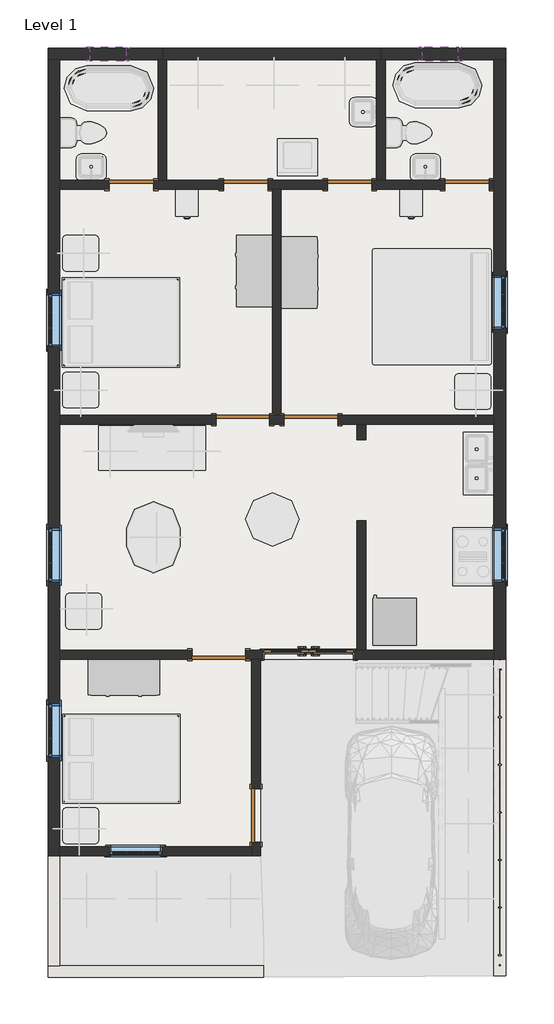
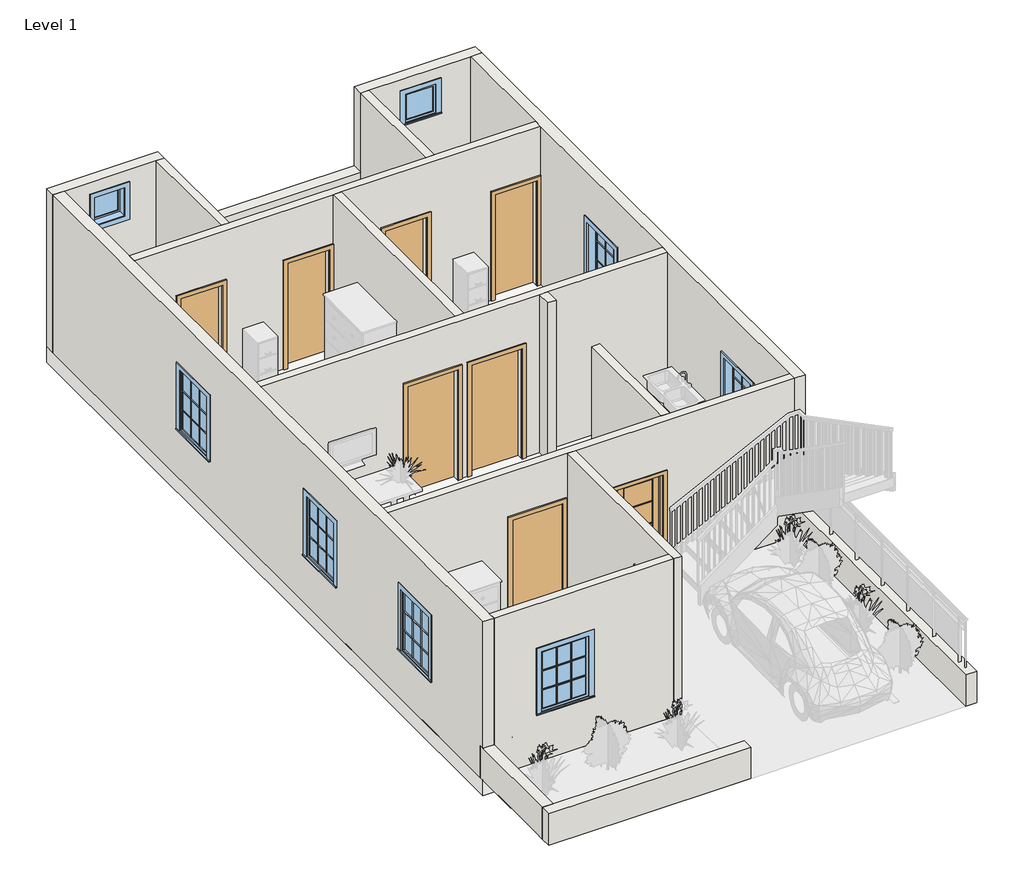
# One storey, part 1 of 3: 18 walls, 9 doors, 8 windows, 1 slab.
"""IFC4 building model written with IfcOpenShell, lengths in millimetres."""

from ifc_helpers import new_model, si_unit, frame, origin, origin_with_axes, place, context, project, spatial, polyline, outline, extrude, faceted_brep, transform, mapped, element, save
from components import door_94998e6c, door_059fdd7e, door_16372e1c, door_686f89d2, window_29c06734, window_5c190c7e, window_e41d21a6

model = new_model("IFC4")

# Units and contexts
model_context = context("Model", 3, world=origin())
ifc_project = project(units=[si_unit("LENGTHUNIT", "METRE", prefix="MILLI")], contexts=[model_context])

# Site, building, storey
site = spatial("IfcSite", under=ifc_project)
building = spatial("IfcBuilding", under=site)
storey = spatial("IfcBuildingStorey", under=building, Name="Level 1", Elevation=0.0)

# Doors
placement = place(None, origin())
door_shape = door_94998e6c(model_context)
element("IfcDoor", 1, ObjectType="Door-Exterior-Double-Full Glass-Wood_Clad : 60\" x 80\"", at=placement, inside=storey, context=model_context, shape_type="MappedRepresentation", body=[
    mapped(door_shape, transform((1366.1339716, 319.025395, 0.0), x_axis=(1.0, 0.0, 0.0), y_axis=(0.0, 1.0, 0.0), z_axis=(0.0, 0.0, 1.0))),
])
door_2_shape = door_059fdd7e(model_context)
element("IfcDoor", 2, ObjectType="Single-Flush : 30\" x 80\"", at=placement, inside=storey, context=model_context, shape_type="MappedRepresentation", body=[
    mapped(door_2_shape, transform((-1669.1660284, 8342.250395, 0.0), x_axis=(1.0, 0.0, 0.0), y_axis=(0.0, 1.0, 0.0), z_axis=(0.0, 0.0, 1.0))),
])
element("IfcDoor", 3, ObjectType="Single-Flush : 30\" x 80\"", at=placement, inside=storey, context=model_context, shape_type="MappedRepresentation", body=[
    mapped(door_2_shape, transform((286.6339716, 8342.250395, 0.0), x_axis=(1.0, 0.0, 0.0), y_axis=(0.0, 1.0, 0.0), z_axis=(0.0, 0.0, 1.0))),
])
element("IfcDoor", 4, ObjectType="Single-Flush : 30\" x 80\"", at=placement, inside=storey, context=model_context, shape_type="MappedRepresentation", body=[
    mapped(door_2_shape, transform((2064.6339716, 8342.250395, 0.0), x_axis=(1.0, 0.0, 0.0), y_axis=(0.0, 1.0, 0.0), z_axis=(0.0, 0.0, 1.0))),
])
element("IfcDoor", 5, ObjectType="Single-Flush : 30\" x 80\"", at=placement, inside=storey, context=model_context, shape_type="MappedRepresentation", body=[
    mapped(door_2_shape, transform((4071.2339716, 8342.250395, 0.0), x_axis=(1.0, 0.0, 0.0), y_axis=(0.0, 1.0, 0.0), z_axis=(0.0, 0.0, 1.0))),
])
door_3_shape = door_16372e1c(model_context)
element("IfcDoor", 6, ObjectType="Single-Flush : 36\" x 84\"", at=placement, inside=storey, context=model_context, shape_type="MappedRepresentation", body=[
    mapped(door_3_shape, transform((235.8339716, 4329.050395, 0.0), x_axis=(1.0, 0.0, 0.0), y_axis=(0.0, 1.0, 0.0), z_axis=(0.0, 0.0, 1.0))),
])
door_4_shape = door_686f89d2(model_context)
element("IfcDoor", 7, ObjectType="Single-Flush : 36\" x 84\"", at=placement, inside=storey, context=model_context, shape_type="MappedRepresentation", body=[
    mapped(door_4_shape, transform((1404.2339716, 4329.050395, 0.0), x_axis=(-1.0, 0.0, 0.0), y_axis=(0.0, -1.0, 0.0), z_axis=(0.0, 0.0, 1.0))),
])
element("IfcDoor", 8, ObjectType="Single-Flush : 36\" x 84\"", at=placement, inside=storey, context=model_context, shape_type="MappedRepresentation", body=[
    mapped(door_4_shape, transform((-170.5660284, 315.850395, 0.0), x_axis=(1.0, 0.0, 0.0), y_axis=(0.0, 1.0, 0.0), z_axis=(0.0, 0.0, 1.0))),
])
element("IfcDoor", 9, ObjectType="Single-Flush : 36\" x 84\"", at=placement, inside=storey, context=model_context, shape_type="MappedRepresentation", body=[
    mapped(door_4_shape, transform((464.4339716, -2427.349605, 0.0), x_axis=(0.0, -1.0, 0.0), y_axis=(1.0, 0.0, 0.0), z_axis=(0.0, 0.0, 1.0))),
])

# Slab
element("IfcSlab", 10, ObjectType="Generic - 12\"", at=placement, inside=storey, context=model_context, shape_type="SweptSolid", body=[
    extrude(outline(polyline([(4731.6339716, 10679.050395), (4731.6339716, 239.650395), (540.6339716, 239.650395), (540.6339716, -3113.149605), (-3091.5660284, -3113.149605), (-3091.5660284, 10679.050395), (4731.6339716, 10679.050395)])), frame((0.0, 0.0, -304.8), z_axis=(0.0, 0.0, 1.0), x_axis=(1.0, 0.0, 0.0)), (0.0, 0.0, 1.0), 304.8),
])

# Walls
element("IfcWall", 11, ObjectType="Generic - 2'", at=placement, inside=storey, context=model_context, shape_type="Brep", body=[
    faceted_brep([(4528.4339716, 315.850395, 0.0), (4528.4339716, 239.650395, 0.0), (4528.4339716, -5170.549605, 0.0), (4528.4339716, -5170.549605, 609.6), (4528.4339716, 315.850395, 609.6), (4731.6339716, 315.850395, 0.0), (4731.6339716, 315.850395, 609.6), (4731.6339716, -5170.549605, 609.6), (4731.6339716, -5170.549605, 0.0)], [[[0, 1, 2, 3, 4]], [[5, 6, 7, 8]], [[2, 1, 0, 5, 8]], [[3, 2, 8, 7]], [[4, 3, 7, 6]], [[0, 4, 6, 5]]]),
])
element("IfcWall", 12, ObjectType="Generic - 2'", at=placement, inside=storey, context=model_context, shape_type="Brep", body=[
    faceted_brep([(591.4339716, -4992.749605, 0.0), (-2888.3660284, -4992.749605, 0.0), (-3091.5660284, -4992.749605, 0.0), (-3091.5660284, -4992.749605, 609.6), (-2888.3660284, -4992.749605, 609.6), (591.4339716, -4992.749605, 609.6), (591.4339716, -5195.949605, 0.0), (591.4339716, -5195.949605, 609.6), (-3091.5660284, -5195.949605, 609.6), (-3091.5660284, -5195.949605, 0.0)], [[[0, 1, 2, 3, 4, 5]], [[6, 7, 8, 9]], [[2, 1, 0, 6, 9]], [[5, 4, 3, 8, 7]], [[0, 5, 7, 6]], [[3, 2, 9, 8]]]),
])
element("IfcWall", 13, ObjectType="Generic - 8\"", at=placement, inside=storey, context=model_context, shape_type="Brep", body=[
    faceted_brep([(-3091.5660284, 10475.850395, 0.0), (-2888.3660284, 10475.850395, 0.0), (-1211.9660284, 10475.850395, 0.0), (-1135.7660284, 10475.850395, 0.0), (-1135.7660284, 10475.850395, 1524.0), (-1059.5660284, 10475.850395, 1524.0), (-1059.5660284, 10475.850395, 3048.0), (-1211.9660284, 10475.850395, 3048.0), (-2888.3660284, 10475.850395, 3048.0), (-3091.5660284, 10475.850395, 3048.0), (-1758.0660284, 10475.850395, 2768.6), (-1758.0660284, 10475.850395, 2159.0), (-2367.6660284, 10475.850395, 2159.0), (-2367.6660284, 10475.850395, 2768.6), (-3091.5660284, 10679.050395, 0.0), (-3091.5660284, 10679.050395, 3048.0), (-1059.5660284, 10679.050395, 3048.0), (-1059.5660284, 10679.050395, 1524.0), (-1135.7660284, 10679.050395, 1524.0), (-1135.7660284, 10679.050395, 0.0), (-1758.0660284, 10679.050395, 2768.6), (-2367.6660284, 10679.050395, 2768.6), (-2367.6660284, 10679.050395, 2159.0), (-1758.0660284, 10679.050395, 2159.0)], [[[0, 1, 2, 3, 4, 5, 6, 7, 8, 9], [10, 11, 12, 13]], [[14, 15, 16, 17, 18, 19], [20, 21, 22, 23]], [[3, 2, 1, 0, 14, 19]], [[0, 9, 15, 14]], [[11, 10, 20, 23]], [[12, 11, 23, 22]], [[13, 12, 22, 21]], [[10, 13, 21, 20]], [[4, 3, 19, 18]], [[17, 5, 4, 18]], [[6, 5, 17, 16]], [[9, 8, 7, 6, 16, 15]]]),
])
element("IfcWall", 14, ObjectType="Generic - 8\"", at=placement, inside=storey, context=model_context, shape_type="Brep", body=[
    faceted_brep([(4528.4339716, 10475.850395, 0.0), (4528.4339716, 8418.450395, 0.0), (4528.4339716, 8266.050395, 0.0), (4528.4339716, 4405.250395, 0.0), (4528.4339716, 4252.850395, 0.0), (4528.4339716, 392.050395, 0.0), (4528.4339716, 315.850395, 0.0), (4528.4339716, 315.850395, 609.6), (4528.4339716, 239.650395, 609.6), (4528.4339716, 239.650395, 3048.0), (4528.4339716, 392.050395, 3048.0), (4528.4339716, 4252.850395, 3048.0), (4528.4339716, 4405.250395, 3048.0), (4528.4339716, 8266.050395, 3048.0), (4528.4339716, 8418.450395, 3048.0), (4528.4339716, 10475.850395, 3048.0), (4528.4339716, 5878.450395, 2133.6), (4528.4339716, 5878.450395, 914.4), (4528.4339716, 6792.850395, 914.4), (4528.4339716, 6792.850395, 2133.6), (4528.4339716, 1560.450395, 2133.6), (4528.4339716, 1560.450395, 914.4), (4528.4339716, 2474.850395, 914.4), (4528.4339716, 2474.850395, 2133.6), (4731.6339716, 10475.850395, 0.0), (4731.6339716, 10475.850395, 3048.0), (4731.6339716, 239.650395, 3048.0), (4731.6339716, 239.650395, 609.6), (4731.6339716, 315.850395, 609.6), (4731.6339716, 315.850395, 0.0), (4731.6339716, 5878.450395, 2133.6), (4731.6339716, 6792.850395, 2133.6), (4731.6339716, 6792.850395, 914.4), (4731.6339716, 5878.450395, 914.4), (4731.6339716, 1560.450395, 2133.6), (4731.6339716, 2474.850395, 2133.6), (4731.6339716, 2474.850395, 914.4), (4731.6339716, 1560.450395, 914.4)], [[[0, 1, 2, 3, 4, 5, 6, 7, 8, 9, 10, 11, 12, 13, 14, 15], [16, 17, 18, 19], [20, 21, 22, 23]], [[24, 25, 26, 27, 28, 29], [30, 31, 32, 33], [34, 35, 36, 37]], [[6, 5, 4, 3, 2, 1, 0, 24, 29]], [[0, 15, 25, 24]], [[7, 6, 29, 28]], [[27, 8, 7, 28]], [[9, 8, 27, 26]], [[17, 16, 30, 33]], [[18, 17, 33, 32]], [[19, 18, 32, 31]], [[16, 19, 31, 30]], [[21, 20, 34, 37]], [[22, 21, 37, 36]], [[23, 22, 36, 35]], [[20, 23, 35, 34]], [[15, 14, 13, 12, 11, 10, 9, 26, 25]]]),
])
element("IfcWall", 15, ObjectType="Generic - 8\"", at=placement, inside=storey, context=model_context, shape_type="Brep", body=[
    faceted_brep([(-2888.3660284, -4992.749605, 0.0), (-2888.3660284, -3113.149605, 0.0), (-2888.3660284, -3036.949605, 0.0), (-2888.3660284, -3036.949605, 609.6), (-2888.3660284, -3113.149605, 609.6), (-2888.3660284, -4992.749605, 609.6), (-3091.5660284, -4992.749605, 0.0), (-3091.5660284, -4992.749605, 609.6), (-3091.5660284, -3113.149605, 609.6), (-3091.5660284, -3036.949605, 609.6), (-3091.5660284, -3036.949605, 0.0)], [[[0, 1, 2, 3, 4, 5]], [[6, 7, 8, 9, 10]], [[2, 1, 0, 6, 10]], [[3, 2, 10, 9]], [[5, 4, 3, 9, 8, 7]], [[0, 5, 7, 6]]]),
])
element("IfcWall", 16, ObjectType="Generic - 8\"", at=placement, inside=storey, context=model_context, shape_type="Brep", body=[
    faceted_brep([(-2888.3660284, -3036.949605, 0.0), (-2888.3660284, -2960.749605, 0.0), (-2888.3660284, 239.650395, 0.0), (-2888.3660284, 392.050395, 0.0), (-2888.3660284, 4252.850395, 0.0), (-2888.3660284, 4405.250395, 0.0), (-2888.3660284, 8266.050395, 0.0), (-2888.3660284, 8418.450395, 0.0), (-2888.3660284, 10475.850395, 0.0), (-2888.3660284, 10475.850395, 3048.0), (-2888.3660284, 8418.450395, 3048.0), (-2888.3660284, 8266.050395, 3048.0), (-2888.3660284, 4405.250395, 3048.0), (-2888.3660284, 4252.850395, 3048.0), (-2888.3660284, 392.050395, 3048.0), (-2888.3660284, 239.650395, 3048.0), (-2888.3660284, -2960.749605, 3048.0), (-2888.3660284, -3113.149605, 3048.0), (-2888.3660284, -3113.149605, 609.6), (-2888.3660284, -3036.949605, 609.6), (-2888.3660284, 6488.050395, 2133.6), (-2888.3660284, 6488.050395, 914.4), (-2888.3660284, 5573.650395, 914.4), (-2888.3660284, 5573.650395, 2133.6), (-2888.3660284, 2474.850395, 2133.6), (-2888.3660284, 2474.850395, 914.4), (-2888.3660284, 1560.450395, 914.4), (-2888.3660284, 1560.450395, 2133.6), (-2888.3660284, -522.349605, 2133.6), (-2888.3660284, -522.349605, 914.4), (-2888.3660284, -1436.749605, 914.4), (-2888.3660284, -1436.749605, 2133.6), (-3091.5660284, -3036.949605, 0.0), (-3091.5660284, -3036.949605, 609.6), (-3091.5660284, -3113.149605, 609.6), (-3091.5660284, -3113.149605, 3048.0), (-3091.5660284, 10475.850395, 3048.0), (-3091.5660284, 10475.850395, 0.0), (-3091.5660284, 6488.050395, 2133.6), (-3091.5660284, 5573.650395, 2133.6), (-3091.5660284, 5573.650395, 914.4), (-3091.5660284, 6488.050395, 914.4), (-3091.5660284, 2474.850395, 2133.6), (-3091.5660284, 1560.450395, 2133.6), (-3091.5660284, 1560.450395, 914.4), (-3091.5660284, 2474.850395, 914.4), (-3091.5660284, -522.349605, 2133.6), (-3091.5660284, -1436.749605, 2133.6), (-3091.5660284, -1436.749605, 914.4), (-3091.5660284, -522.349605, 914.4)], [[[0, 1, 2, 3, 4, 5, 6, 7, 8, 9, 10, 11, 12, 13, 14, 15, 16, 17, 18, 19], [20, 21, 22, 23], [24, 25, 26, 27], [28, 29, 30, 31]], [[32, 33, 34, 35, 36, 37], [38, 39, 40, 41], [42, 43, 44, 45], [46, 47, 48, 49]], [[8, 7, 6, 5, 4, 3, 2, 1, 0, 32, 37]], [[9, 8, 37, 36]], [[0, 19, 33, 32]], [[18, 34, 33, 19]], [[18, 17, 35, 34]], [[21, 20, 38, 41]], [[22, 21, 41, 40]], [[23, 22, 40, 39]], [[20, 23, 39, 38]], [[25, 24, 42, 45]], [[26, 25, 45, 44]], [[27, 26, 44, 43]], [[24, 27, 43, 42]], [[29, 28, 46, 49]], [[30, 29, 49, 48]], [[31, 30, 48, 47]], [[28, 31, 47, 46]], [[17, 16, 15, 14, 13, 12, 11, 10, 9, 36, 35]]]),
])
element("IfcWall", 17, ObjectType="Generic - 8\"", at=placement, inside=storey, context=model_context, shape_type="Brep", body=[
    faceted_brep([(2598.0339716, 10475.850395, 0.0), (2674.2339716, 10475.850395, 0.0), (4528.4339716, 10475.850395, 0.0), (4731.6339716, 10475.850395, 0.0), (4731.6339716, 10475.850395, 3048.0), (4528.4339716, 10475.850395, 3048.0), (2674.2339716, 10475.850395, 3048.0), (2521.8339716, 10475.850395, 3048.0), (2521.8339716, 10475.850395, 1524.0), (2598.0339716, 10475.850395, 1524.0), (3309.2339716, 10475.850395, 2768.6), (3918.8339716, 10475.850395, 2768.6), (3918.8339716, 10475.850395, 2159.0), (3309.2339716, 10475.850395, 2159.0), (2598.0339716, 10679.050395, 0.0), (2598.0339716, 10679.050395, 1524.0), (2521.8339716, 10679.050395, 1524.0), (2521.8339716, 10679.050395, 3048.0), (4731.6339716, 10679.050395, 3048.0), (4731.6339716, 10679.050395, 0.0), (3309.2339716, 10679.050395, 2768.6), (3309.2339716, 10679.050395, 2159.0), (3918.8339716, 10679.050395, 2159.0), (3918.8339716, 10679.050395, 2768.6)], [[[0, 1, 2, 3, 4, 5, 6, 7, 8, 9], [10, 11, 12, 13]], [[14, 15, 16, 17, 18, 19], [20, 21, 22, 23]], [[3, 2, 1, 0, 14, 19]], [[4, 3, 19, 18]], [[20, 23, 11, 10]], [[23, 22, 12, 11]], [[22, 21, 13, 12]], [[21, 20, 10, 13]], [[0, 9, 15, 14]], [[8, 16, 15, 9]], [[8, 7, 17, 16]], [[7, 6, 5, 4, 18, 17]]]),
])
element("IfcWall", 18, ObjectType="Generic - 8\"", at=placement, inside=storey, context=model_context, shape_type="Brep", body=[
    faceted_brep([(-1135.7660284, 10475.850395, 0.0), (-1059.5660284, 10475.850395, 0.0), (2521.8339716, 10475.850395, 0.0), (2598.0339716, 10475.850395, 0.0), (2598.0339716, 10475.850395, 1524.0), (2521.8339716, 10475.850395, 1524.0), (-1059.5660284, 10475.850395, 1524.0), (-1135.7660284, 10475.850395, 1524.0), (-1135.7660284, 10679.050395, 0.0), (-1135.7660284, 10679.050395, 1524.0), (-1059.5660284, 10679.050395, 1524.0), (2521.8339716, 10679.050395, 1524.0), (2598.0339716, 10679.050395, 1524.0), (2598.0339716, 10679.050395, 0.0)], [[[0, 1, 2, 3, 4, 5, 6, 7]], [[8, 9, 10, 11, 12, 13]], [[3, 2, 1, 0, 8, 13]], [[4, 3, 13, 12]], [[7, 6, 5, 4, 12, 11, 10, 9]], [[0, 7, 9, 8]]]),
])
element("IfcWall", 19, ObjectType="INNER 6\"", at=placement, inside=storey, context=model_context, shape_type="Brep", body=[
    faceted_brep([(4452.2339716, 8266.050395, 2032.0), (4452.2339716, 8266.050395, 0.0), (4528.4339716, 8266.050395, 0.0), (4528.4339716, 8266.050395, 3048.0), (896.2339716, 8266.050395, 3048.0), (743.8339716, 8266.050395, 3048.0), (-2888.3660284, 8266.050395, 3048.0), (-2888.3660284, 8266.050395, 0.0), (-2050.1660284, 8266.050395, 0.0), (-2050.1660284, 8266.050395, 2032.0), (-1288.1660284, 8266.050395, 2032.0), (-1288.1660284, 8266.050395, 0.0), (-94.3660284, 8266.050395, 0.0), (-94.3660284, 8266.050395, 2032.0), (667.6339716, 8266.050395, 2032.0), (667.6339716, 8266.050395, 0.0), (743.8339716, 8266.050395, 0.0), (896.2339716, 8266.050395, 0.0), (1683.6339716, 8266.050395, 0.0), (1683.6339716, 8266.050395, 2032.0), (2445.6339716, 8266.050395, 2032.0), (2445.6339716, 8266.050395, 0.0), (3690.2339716, 8266.050395, 0.0), (3690.2339716, 8266.050395, 2032.0), (4528.4339716, 8418.450395, 0.0), (4452.2339716, 8418.450395, 0.0), (4452.2339716, 8418.450395, 2032.0), (3690.2339716, 8418.450395, 2032.0), (3690.2339716, 8418.450395, 0.0), (2674.2339716, 8418.450395, 0.0), (2521.8339716, 8418.450395, 0.0), (2445.6339716, 8418.450395, 0.0), (2445.6339716, 8418.450395, 2032.0), (1683.6339716, 8418.450395, 2032.0), (1683.6339716, 8418.450395, 0.0), (667.6339716, 8418.450395, 0.0), (667.6339716, 8418.450395, 2032.0), (-94.3660284, 8418.450395, 2032.0), (-94.3660284, 8418.450395, 0.0), (-1059.5660284, 8418.450395, 0.0), (-1211.9660284, 8418.450395, 0.0), (-1288.1660284, 8418.450395, 0.0), (-1288.1660284, 8418.450395, 2032.0), (-2050.1660284, 8418.450395, 2032.0), (-2050.1660284, 8418.450395, 0.0), (-2888.3660284, 8418.450395, 0.0), (-2888.3660284, 8418.450395, 3048.0), (-1211.9660284, 8418.450395, 3048.0), (-1059.5660284, 8418.450395, 3048.0), (2521.8339716, 8418.450395, 3048.0), (2674.2339716, 8418.450395, 3048.0), (4528.4339716, 8418.450395, 3048.0)], [[[0, 1, 2, 3, 4, 5, 6, 7, 8, 9, 10, 11, 12, 13, 14, 15, 16, 17, 18, 19, 20, 21, 22, 23]], [[24, 25, 26, 27, 28, 29, 30, 31, 32, 33, 34, 35, 36, 37, 38, 39, 40, 41, 42, 43, 44, 45, 46, 47, 48, 49, 50, 51]], [[8, 7, 45, 44]], [[12, 11, 41, 40, 39, 38]], [[18, 17, 16, 15, 35, 34]], [[22, 21, 31, 30, 29, 28]], [[2, 1, 25, 24]], [[3, 2, 24, 51]], [[7, 6, 46, 45]], [[42, 41, 11, 10]], [[43, 42, 10, 9]], [[44, 43, 9, 8]], [[36, 35, 15, 14]], [[37, 36, 14, 13]], [[38, 37, 13, 12]], [[32, 31, 21, 20]], [[33, 32, 20, 19]], [[34, 33, 19, 18]], [[26, 25, 1, 0]], [[27, 26, 0, 23]], [[28, 27, 23, 22]], [[6, 5, 4, 3, 51, 50, 49, 48, 47, 46]]]),
])
element("IfcWall", 20, ObjectType="INNER 6\"", at=placement, inside=storey, context=model_context, shape_type="Brep", body=[
    faceted_brep([(693.0339716, 4252.850395, 0.0), (947.0339716, 4252.850395, 0.0), (947.0339716, 4252.850395, 2133.6), (1861.4339716, 4252.850395, 2133.6), (1861.4339716, 4252.850395, 0.0), (2191.6339716, 4252.850395, 0.0), (2344.0339716, 4252.850395, 0.0), (4528.4339716, 4252.850395, 0.0), (4528.4339716, 4252.850395, 3048.0), (2344.0339716, 4252.850395, 3048.0), (2191.6339716, 4252.850395, 3048.0), (-2888.3660284, 4252.850395, 3048.0), (-2888.3660284, 4252.850395, 0.0), (-221.3660284, 4252.850395, 0.0), (-221.3660284, 4252.850395, 2133.6), (693.0339716, 4252.850395, 2133.6), (947.0339716, 4405.250395, 2133.6), (947.0339716, 4405.250395, 0.0), (896.2339716, 4405.250395, 0.0), (743.8339716, 4405.250395, 0.0), (693.0339716, 4405.250395, 0.0), (693.0339716, 4405.250395, 2133.6), (-221.3660284, 4405.250395, 2133.6), (-221.3660284, 4405.250395, 0.0), (-2888.3660284, 4405.250395, 0.0), (-2888.3660284, 4405.250395, 3048.0), (743.8339716, 4405.250395, 3048.0), (896.2339716, 4405.250395, 3048.0), (4528.4339716, 4405.250395, 3048.0), (4528.4339716, 4405.250395, 0.0), (1861.4339716, 4405.250395, 0.0), (1861.4339716, 4405.250395, 2133.6)], [[[0, 1, 2, 3, 4, 5, 6, 7, 8, 9, 10, 11, 12, 13, 14, 15]], [[16, 17, 18, 19, 20, 21, 22, 23, 24, 25, 26, 27, 28, 29, 30, 31]], [[13, 12, 24, 23]], [[30, 29, 7, 6, 5, 4]], [[20, 19, 18, 17, 1, 0]], [[8, 7, 29, 28]], [[12, 11, 25, 24]], [[21, 20, 0, 15]], [[22, 21, 15, 14]], [[23, 22, 14, 13]], [[2, 1, 17, 16]], [[3, 2, 16, 31]], [[4, 3, 31, 30]], [[11, 10, 9, 8, 28, 27, 26, 25]]]),
])
element("IfcWall", 21, ObjectType="INNER 6\"", at=placement, inside=storey, context=model_context, shape_type="SweptSolid", body=[
    extrude(outline(polyline([(743.8339716, 4405.250395), (743.8339716, 8266.050395), (896.2339716, 8266.050395), (896.2339716, 4405.250395), (743.8339716, 4405.250395)])), origin_with_axes(), (0.0, 0.0, 1.0), 3048.0),
])
element("IfcWall", 22, ObjectType="INNER 6\"", at=placement, inside=storey, context=model_context, shape_type="SweptSolid", body=[
    extrude(outline(polyline([(2191.6339716, 3986.150395), (2191.6339716, 4252.850395), (2344.0339716, 4252.850395), (2344.0339716, 3986.150395), (2191.6339716, 3986.150395)])), origin_with_axes(), (0.0, 0.0, 1.0), 3048.0),
])
element("IfcWall", 23, ObjectType="INNER 6\"", at=placement, inside=storey, context=model_context, shape_type="Brep", body=[
    faceted_brep([(-2888.3660284, 239.650395, 3048.0), (-2888.3660284, 239.650395, 0.0), (-627.7660284, 239.650395, 0.0), (-627.7660284, 239.650395, 2133.6), (286.6339716, 239.650395, 2133.6), (286.6339716, 239.650395, 0.0), (388.2339716, 239.650395, 0.0), (540.6339716, 239.650395, 0.0), (578.7339716, 239.650395, 0.0), (578.7339716, 239.650395, 2057.4), (2153.5339716, 239.650395, 2057.4), (2153.5339716, 239.650395, 0.0), (4528.4339716, 239.650395, 0.0), (4528.4339716, 239.650395, 609.6), (4528.4339716, 239.650395, 3048.0), (540.6339716, 239.650395, 3048.0), (388.2339716, 239.650395, 3048.0), (-2888.3660284, 392.050395, 3048.0), (2191.6339716, 392.050395, 3048.0), (2344.0339716, 392.050395, 3048.0), (4528.4339716, 392.050395, 3048.0), (4528.4339716, 392.050395, 0.0), (2344.0339716, 392.050395, 0.0), (2191.6339716, 392.050395, 0.0), (2153.5339716, 392.050395, 0.0), (2153.5339716, 392.050395, 2057.4), (578.7339716, 392.050395, 2057.4), (578.7339716, 392.050395, 0.0), (286.6339716, 392.050395, 0.0), (286.6339716, 392.050395, 2133.6), (-627.7660284, 392.050395, 2133.6), (-627.7660284, 392.050395, 0.0), (-2888.3660284, 392.050395, 0.0), (4528.4339716, 315.850395, 0.0)], [[[0, 1, 2, 3, 4, 5, 6, 7, 8, 9, 10, 11, 12, 13, 14, 15, 16]], [[17, 18, 19, 20, 21, 22, 23, 24, 25, 26, 27, 28, 29, 30, 31, 32]], [[1, 32, 31, 2]], [[5, 28, 27, 8, 7, 6]], [[21, 33, 12, 11, 24, 23, 22]], [[1, 0, 17, 32]], [[29, 28, 5, 4]], [[30, 29, 4, 3]], [[31, 30, 3, 2]], [[12, 33, 21, 20, 14, 13]], [[10, 25, 24, 11]], [[25, 10, 9, 26]], [[26, 9, 8, 27]], [[20, 19, 18, 17, 0, 16, 15, 14]]]),
])
element("IfcWall", 24, ObjectType="INNER 6\"", at=placement, inside=storey, context=model_context, shape_type="Brep", body=[
    faceted_brep([(388.2339716, -2884.549605, 2133.6), (388.2339716, -2884.549605, 0.0), (388.2339716, -2960.749605, 0.0), (388.2339716, -3113.149605, 0.0), (388.2339716, -3113.149605, 3048.0), (388.2339716, -2960.749605, 3048.0), (388.2339716, 239.650395, 3048.0), (388.2339716, 239.650395, 0.0), (388.2339716, -1970.149605, 0.0), (388.2339716, -1970.149605, 2133.6), (540.6339716, -3113.149605, 0.0), (540.6339716, -2884.549605, 0.0), (540.6339716, -2884.549605, 2133.6), (540.6339716, -1970.149605, 2133.6), (540.6339716, -1970.149605, 0.0), (540.6339716, 239.650395, 0.0), (540.6339716, 239.650395, 3048.0), (540.6339716, -3113.149605, 3048.0)], [[[0, 1, 2, 3, 4, 5, 6, 7, 8, 9]], [[10, 11, 12, 13, 14, 15, 16, 17]], [[8, 7, 15, 14]], [[3, 2, 1, 11, 10]], [[7, 6, 16, 15]], [[4, 3, 10, 17]], [[12, 11, 1, 0]], [[13, 12, 0, 9]], [[14, 13, 9, 8]], [[6, 5, 4, 17, 16]]]),
])
element("IfcWall", 25, ObjectType="INNER 6\"", at=placement, inside=storey, context=model_context, shape_type="Brep", body=[
    faceted_brep([(388.2339716, -2960.749605, 0.0), (-2888.3660284, -2960.749605, 0.0), (-2888.3660284, -2960.749605, 3048.0), (388.2339716, -2960.749605, 3048.0), (-2050.1660284, -2960.749605, 2133.6), (-2050.1660284, -2960.749605, 914.4), (-1135.7660284, -2960.749605, 914.4), (-1135.7660284, -2960.749605, 2133.6), (388.2339716, -3113.149605, 0.0), (388.2339716, -3113.149605, 3048.0), (-2888.3660284, -3113.149605, 3048.0), (-2888.3660284, -3113.149605, 609.6), (-2888.3660284, -3113.149605, 0.0), (-2050.1660284, -3113.149605, 2133.6), (-1135.7660284, -3113.149605, 2133.6), (-1135.7660284, -3113.149605, 914.4), (-2050.1660284, -3113.149605, 914.4), (-2888.3660284, -3036.949605, 0.0)], [[[0, 1, 2, 3], [4, 5, 6, 7]], [[8, 9, 10, 11, 12], [13, 14, 15, 16]], [[1, 0, 8, 12, 17]], [[0, 3, 9, 8]], [[1, 17, 12, 11, 10, 2]], [[5, 4, 13, 16]], [[6, 5, 16, 15]], [[7, 6, 15, 14]], [[4, 7, 14, 13]], [[3, 2, 10, 9]]]),
])
element("IfcWall", 26, ObjectType="INNER 6\"", at=placement, inside=storey, context=model_context, shape_type="Brep", body=[
    faceted_brep([(-1211.9660284, 10475.850395, 3048.0), (-1211.9660284, 10475.850395, 0.0), (-1211.9660284, 8418.450395, 0.0), (-1211.9660284, 8418.450395, 3048.0), (-1059.5660284, 10475.850395, 0.0), (-1059.5660284, 10475.850395, 1524.0), (-1059.5660284, 10475.850395, 3048.0), (-1059.5660284, 8418.450395, 3048.0), (-1059.5660284, 8418.450395, 0.0), (-1135.7660284, 10475.850395, 0.0)], [[[0, 1, 2, 3]], [[4, 5, 6, 7, 8]], [[2, 1, 9, 4, 8]], [[3, 2, 8, 7]], [[0, 6, 5, 4, 9, 1]], [[0, 3, 7, 6]]]),
])
element("IfcWall", 27, ObjectType="INNER 6\"", at=placement, inside=storey, context=model_context, shape_type="Brep", body=[
    faceted_brep([(2521.8339716, 10475.850395, 3048.0), (2521.8339716, 10475.850395, 1524.0), (2521.8339716, 10475.850395, 0.0), (2521.8339716, 8418.450395, 0.0), (2521.8339716, 8418.450395, 3048.0), (2674.2339716, 10475.850395, 0.0), (2674.2339716, 10475.850395, 3048.0), (2674.2339716, 8418.450395, 3048.0), (2674.2339716, 8418.450395, 0.0), (2598.0339716, 10475.850395, 0.0)], [[[0, 1, 2, 3, 4]], [[5, 6, 7, 8]], [[3, 2, 9, 5, 8]], [[4, 3, 8, 7]], [[0, 6, 5, 9, 2, 1]], [[0, 4, 7, 6]]]),
])
element("IfcWall", 28, ObjectType="INNER 6\"", at=placement, inside=storey, context=model_context, shape_type="SweptSolid", body=[
    extrude(outline(polyline([(2191.6339716, 392.050395), (2191.6339716, 2601.850395), (2344.0339716, 2601.850395), (2344.0339716, 392.050395), (2191.6339716, 392.050395)])), origin_with_axes(), (0.0, 0.0, 1.0), 3048.0),
])

# Windows
window_shape = window_29c06734(model_context)
element("IfcWindow", 29, ObjectType="Casement 3x3 with Trim : 36\" x 48\"", at=placement, inside=storey, context=model_context, shape_type="MappedRepresentation", body=[
    mapped(window_shape, transform((-2989.9660284, 6030.850395, 0.0), x_axis=(0.0, 1.0, 0.0), y_axis=(-1.0, 0.0, 0.0), z_axis=(0.0, 0.0, 1.0))),
])
element("IfcWindow", 30, ObjectType="Casement 3x3 with Trim : 36\" x 48\"", at=placement, inside=storey, context=model_context, shape_type="MappedRepresentation", body=[
    mapped(window_shape, transform((4630.0339716, 6335.650395, 0.0), x_axis=(0.0, -1.0, 0.0), y_axis=(1.0, 0.0, 0.0), z_axis=(0.0, 0.0, 1.0))),
])
element("IfcWindow", 31, ObjectType="Casement 3x3 with Trim : 36\" x 48\"", at=placement, inside=storey, context=model_context, shape_type="MappedRepresentation", body=[
    mapped(window_shape, transform((-2989.9660284, 2017.650395, 0.0), x_axis=(0.0, 1.0, 0.0), y_axis=(-1.0, 0.0, 0.0), z_axis=(0.0, 0.0, 1.0))),
])
element("IfcWindow", 32, ObjectType="Casement 3x3 with Trim : 36\" x 48\"", at=placement, inside=storey, context=model_context, shape_type="MappedRepresentation", body=[
    mapped(window_shape, transform((4630.0339716, 2017.650395, 0.0), x_axis=(0.0, -1.0, 0.0), y_axis=(1.0, 0.0, 0.0), z_axis=(0.0, 0.0, 1.0))),
])
element("IfcWindow", 33, ObjectType="Casement 3x3 with Trim : 36\" x 48\"", at=placement, inside=storey, context=model_context, shape_type="MappedRepresentation", body=[
    mapped(window_shape, transform((-2989.9660284, -979.549605, 0.0), x_axis=(0.0, 1.0, 0.0), y_axis=(-1.0, 0.0, 0.0), z_axis=(0.0, 0.0, 1.0))),
])
window_2_shape = window_5c190c7e(model_context)
element("IfcWindow", 34, ObjectType="Casement 3x3 with Trim : 36\" x 48\"", at=placement, inside=storey, context=model_context, shape_type="MappedRepresentation", body=[
    mapped(window_2_shape, transform((-1592.9660284, -3036.949605, 0.0), x_axis=(-1.0, 0.0, 0.0), y_axis=(0.0, -1.0, 0.0), z_axis=(0.0, 0.0, 1.0))),
])
window_3_shape = window_e41d21a6(model_context)
element("IfcWindow", 35, ObjectType="Transom with Trim : 24\" x 24\"", at=placement, inside=storey, context=model_context, shape_type="MappedRepresentation", body=[
    mapped(window_3_shape, transform((-2024.7660284, 10577.450395, 0.0), x_axis=(1.0, 0.0, 0.0), y_axis=(0.0, 1.0, 0.0), z_axis=(0.0, 0.0, 1.0))),
])
element("IfcWindow", 36, ObjectType="Transom with Trim : 24\" x 24\"", at=placement, inside=storey, context=model_context, shape_type="MappedRepresentation", body=[
    mapped(window_3_shape, transform((3575.9339716, 10577.450395, 0.0), x_axis=(-1.0, 0.0, 0.0), y_axis=(0.0, -1.0, 0.0), z_axis=(0.0, 0.0, 1.0))),
])

save(model, "model.ifc")

# Revit data of these elements
# Type "Door-Exterior-Double-Full Glass-Wood_Clad : 60\" x 80\""
#   Type Mark = "8"
#   Assembly Code = "B2030100"
#   Analytic Construction = "French door, wood frame with double glass"
#   Top Rail = 0' - 4 11/16"
#   Threshold Offset [instance default] = 0' - 0 1/2"
#   Thickness = 0' - 1 3/8"
#   Thermal Resistance (R) = 1.9158 (h·ft²·°F)/BTU
#   Swing Angle [instance default] = 90.00°
#   Stiles = 0' - 4 3/4"
#   Rough Width = 5' - 2"
#   Rough Height = 6' - 9"
#   Panel Width = 2' - 6"
#   Door Offset [instance default] = 0' - 0"
#   Height = 6' - 8"
#   Width = 5' - 0"
#   Heat Transfer Coefficient (U) = 0.5220 BTU/(h·ft²·°F)
#   Bottom Rail = 0' - 9 1/8"
#   Exterior Trim [instance default] = yes
#   Threshold [instance default] = yes
#   Show Grill [instance default] = yes
#   Function = 1
#   Trim Material = Cherry
#   Threshold Material = Cherry
#   Panel Material = Cherry
#   Glazing = Glass
#   Frame Material = Cherry
#   Door Handle Material = Aluminum
#   Visual Light Transmittance = 0
#   Solar Heat Gain Coefficient = 0
#   Wall Closure = (empty or 0)
#   Construction Type = (empty or 0)
# Type "Single-Flush : 30\" x 80\""
#   Type Mark = "5"
#   Construction Type Id = "MDOOR"
#   Assembly Code = "C1020"
#   Analytic Construction = "Metal"
#   Thickness = 0' - 2"
#   Heat Transfer Coefficient (U) = 0.651978 BTU/(h·ft²·°F)
#   Height = 6' - 8"
#   Trim Projection Ext = 0' - 1"
#   Trim Projection Int = 0' - 1"
#   Trim Width = 0' - 3"
#   Width = 2' - 6"
#   Define Thermal Properties by = 1
#   Door Material = Door - Panel
#   Frame Material = Door - Frame
#   Visual Light Transmittance = 0
#   Solar Heat Gain Coefficient = 0
#   Function = (empty or 0)
#   Wall Closure = (empty or 0)
# Type "Single-Flush : 36\" x 84\""
#   Type Mark = "1"
#   Construction Type Id = "MDOOR"
#   Assembly Code = "C1020"
#   Analytic Construction = "Metal"
#   Thickness = 0' - 2"
#   Heat Transfer Coefficient (U) = 0.651978 BTU/(h·ft²·°F)
#   Height = 7' - 0"
#   Trim Projection Ext = 0' - 1"
#   Trim Projection Int = 0' - 1"
#   Trim Width = 0' - 3"
#   Width = 3' - 0"
#   Define Thermal Properties by = 1
#   Door Material = Door - Panel
#   Frame Material = Door - Frame
#   Visual Light Transmittance = 0
#   Solar Heat Gain Coefficient = 0
#   Function = (empty or 0)
#   Wall Closure = (empty or 0)
# Type "Generic - 12\""
#   Assembly Code = "B1010"
#   Function = 0
#   Layers, outside or top first: 1' - 0" no material (function 1)
# Type "Generic - 2'"
#   Assembly Code = "B2010"
#   Layers, outside or top first: 0' - 8" "Birch" (function 1)
# Type "Generic - 8\""
#   Assembly Code = "B2010"
#   Layers, outside or top first: 0' - 8" "Brick, Common" (function 1)
# Type "INNER 6\""
#   Assembly Code = "B2010"
#   Layers, outside or top first: 0' - 6" "Brick, Common" (function 1)
# Type "Casement 3x3 with Trim : 36\" x 48\""
#   Type Mark = "10"
#   Construction Type Id = "GSP4R"
#   Assembly Code = "B2020100"
#   Analytic Construction = "1/8 in Pilkington single glazing"
#   Visual Light Transmittance = 0.9
#   Solar Heat Gain Coefficient = 0.78
#   Heat Transfer Coefficient (U) = 0.6496 BTU/(h·ft²·°F)
#   Height = 4' - 0"
#   Default Sill Height = 3' - 0"
#   Trim Projection - Ext. = 0' - 0 1/2"
#   Trim Projection - Int. = 0' - 0 3/4"
#   Trim Width - Exterior = 0' - 3 1/2"
#   Trim Width - Interior = 0' - 3 1/2"
#   Width = 3' - 0"
#   Window Inset = 0' - 0 3/4"
#   Define Thermal Properties by = 1
#   Glass Pane Material = Glass
#   Sash Material = Sash
#   Trim Exterior Material = Trim
#   Trim Interior Material = Trim
#   Wall Closure = (empty or 0)
# Type "Transom with Trim : 24\" x 24\""
#   Type Mark = "13"
#   Construction Type Id = "GSP4R"
#   Assembly Code = "B2020100"
#   Analytic Construction = "1/8 in Pilkington single glazing"
#   Visual Light Transmittance = 0.9
#   Solar Heat Gain Coefficient = 0.78
#   Heat Transfer Coefficient (U) = 0.6496 BTU/(h·ft²·°F)
#   Height = 2' - 0"
#   Default Sill Height = 7' - 1"
#   Trim Projection - Ext. = 0' - 0 1/2"
#   Trim Projection - Int. = 0' - 0 3/4"
#   Trim Width - Exterior = 0' - 3 1/2"
#   Trim Width - Interior = 0' - 3 1/2"
#   Width = 2' - 0"
#   Window Inset = 0' - 0 3/4"
#   Define Thermal Properties by = 1
#   Glass Pane Material = Glass
#   Sash Material = Sash
#   Trim Exterior Material = Trim
#   Trim Interior Material = Trim
#   Wall Closure = (empty or 0)
# Element 1 (IfcDoor, "Door-Exterior-Double-Full Glass-Wood_Clad : 60\" x 80\"")
#   Threshold Offset = 0' - 0 1/2"
#   Swing Angle = 90.00°
#   Door Offset = 0' - 0"
#   Threshold = yes
#   Show Grill = yes
#   Exterior Trim = yes
#   Phase Created = New Construction
#   Materials on its faces: "Cherry", "Aluminum", "Glass"
# Elements 2, 3, 4, 5 (IfcDoor, "Single-Flush : 30\" x 80\"")
#   Phase Created = New Construction
#   Materials on its faces: "Door - Frame", "Door - Panel"
# Elements 6, 7, 8, 9 (IfcDoor, "Single-Flush : 36\" x 84\"")
#   Phase Created = New Construction
#   Materials on its faces: "Door - Frame", "Door - Panel"
# Element 10 (IfcSlab, "Generic - 12\"")
#   Height Offset From Level = 0' - 0"
#   Phase Created = New Construction
#   Materials on its faces: "Default Floor"
# Element 11 (IfcWall, "Generic - 2'")
#   Top Offset = 0' - 0"
#   Base Offset = 0' - 0"
#   Unconnected Height = 2' - 0"
#   wall height = 2' - 0"
#   Phase Created = New Construction
#   Base Constraint = Level 1
#   Materials on its faces: "Birch"
# Element 12 (IfcWall, "Generic - 2'")
#   Top Offset = 0' - 0"
#   Base Offset = 0' - 0"
#   Unconnected Height = 2' - 0"
#   wall height = 2' - 0"
#   Phase Created = New Construction
#   Base Constraint = Level 1
#   Materials on its faces: "Birch", "Brick, Common"
# Elements 13, 14, 16, 17 (IfcWall, "Generic - 8\"")
#   Top Offset = 0' - 0"
#   Base Offset = 0' - 0"
#   Unconnected Height = 10' - 0"
#   wall height = 10' - 0"
#   Phase Created = New Construction
#   Base Constraint = Level 1
#   Materials on its faces: "Brick, Common"
# Element 15 (IfcWall, "Generic - 8\"")
#   Top Offset = 0' - 0"
#   Base Offset = 0' - 0"
#   Unconnected Height = 2' - 0"
#   wall height = 2' - 0"
#   Phase Created = New Construction
#   Base Constraint = Level 1
#   Materials on its faces: "Brick, Common"
# Element 18 (IfcWall, "Generic - 8\"")
#   Top Offset = 0' - 0"
#   Base Offset = 0' - 0"
#   Unconnected Height = 5' - 0"
#   wall height = 5' - 0"
#   Phase Created = New Construction
#   Base Constraint = Level 1
#   Materials on its faces: "Brick, Common"
# Elements 19, 20, 21, 22, 23, 24, 25, 26, 27, 28 (IfcWall, "INNER 6\"")
#   Top Offset = 0' - 0"
#   Base Offset = 0' - 0"
#   Unconnected Height = 10' - 0"
#   wall height = 10' - 0"
#   Phase Created = New Construction
#   Base Constraint = Level 1
#   Materials on its faces: "Brick, Common"
# Element 29 (IfcWindow, "Casement 3x3 with Trim : 36\" x 48\"")
#   Mark = "1"
#   Phase Created = New Construction
#   Materials on its faces: "Sash", "Glass", "Trim"
# Element 30 (IfcWindow, "Casement 3x3 with Trim : 36\" x 48\"")
#   Mark = "2"
#   Phase Created = New Construction
#   Materials on its faces: "Sash", "Glass", "Trim"
# Element 31 (IfcWindow, "Casement 3x3 with Trim : 36\" x 48\"")
#   Mark = "3"
#   Phase Created = New Construction
#   Materials on its faces: "Sash", "Glass", "Trim"
# Element 32 (IfcWindow, "Casement 3x3 with Trim : 36\" x 48\"")
#   Mark = "4"
#   Phase Created = New Construction
#   Materials on its faces: "Sash", "Glass", "Trim"
# Element 33 (IfcWindow, "Casement 3x3 with Trim : 36\" x 48\"")
#   Mark = "6"
#   Phase Created = New Construction
#   Materials on its faces: "Sash", "Glass", "Trim"
# Element 34 (IfcWindow, "Casement 3x3 with Trim : 36\" x 48\"")
#   Mark = "5"
#   Phase Created = New Construction
#   Materials on its faces: "Sash", "Glass", "Trim"
# Element 35 (IfcWindow, "Transom with Trim : 24\" x 24\"")
#   Mark = "7"
#   Phase Created = New Construction
#   Materials on its faces: "Sash", "Trim", "Glass"
# Element 36 (IfcWindow, "Transom with Trim : 24\" x 24\"")
#   Mark = "8"
#   Phase Created = New Construction
#   Materials on its faces: "Sash", "Trim", "Glass"
# Materials
#   "Cherry": class "Wood", colour RGB 226 177 128, transparency 0, Description = "Prunus Serotina", Cost = 0
#   "Glass": class "Glass", colour RGB 0 128 192, transparency 0.75, Description = "Soda Lime Glass", Cost = 0
#   "Aluminum": class "Metal", colour RGB 247 247 247, transparency 0, Description = "Aluminum 6061", Cost = 0
#   "Door - Panel": class "Wood", colour RGB 210 159 95, transparency 0
#   "Door - Frame": colour RGB 118 70 51, transparency 0
#   "Birch": class "Wood", colour RGB 224 178 126, transparency 0, Description = "Betula Alleghaniensis", Cost = 0
#   "Brick, Common": class "Masonry", colour RGB 170 98 104, transparency 0, Description = "Common brick", Cost = 0
#   "Sash": class "Wood", colour RGB 224 178 126, transparency 0
#   "Trim": class "Wood", colour RGB 224 178 126, transparency 0
#   "Default Floor": colour RGB 128 128 128, transparency 0
# Room at (-2080.423, 9462.331) mm, phase "New Construction", upper level "Level 1", upper offset 10' - 0", lower offset 0' - 0"
#   Number = "1"
#   Name = "BATH"
# Room at (783.923, 9462.331) mm, phase "New Construction", upper level "Level 1", upper offset 10' - 0", lower offset 0' - 0"
#   Number = "3"
# Room at (-993.832, 6196.416) mm, phase "New Construction", upper level "Level 1", upper offset 10' - 0", lower offset 0' - 0"
#   Number = "4"
#   Name = "GUEST ROOM"
# Room at (2647.479, 6196.416) mm, phase "New Construction", upper level "Level 1", upper offset 10' - 0", lower offset 0' - 0"
#   Number = "5"
# Room at (-1581.321, -1507.399) mm, phase "New Construction", upper level "Level 1", upper offset 10' - 0", lower offset 0' - 0"
#   Number = "8"
#   Name = "BEDROOM"
# Room at (3364.407, 2284.631) mm, phase "New Construction", upper level "Level 1", upper offset 10' - 0", lower offset 0' - 0"
#   Number = "6"
#   Name = "KITCHEN"
# Room at (3590.195, 9462.331) mm, phase "New Construction", upper level "Level 1", upper offset 10' - 0", lower offset 0' - 0"
#   Number = "2"
#   Name = "BATH"
# Room at (-993.56, 2284.631) mm, phase "New Construction", upper level "Level 1", upper offset 10' - 0", lower offset 0' - 0"
#   Number = "7"
#   Name = "LIVING/DINING"
